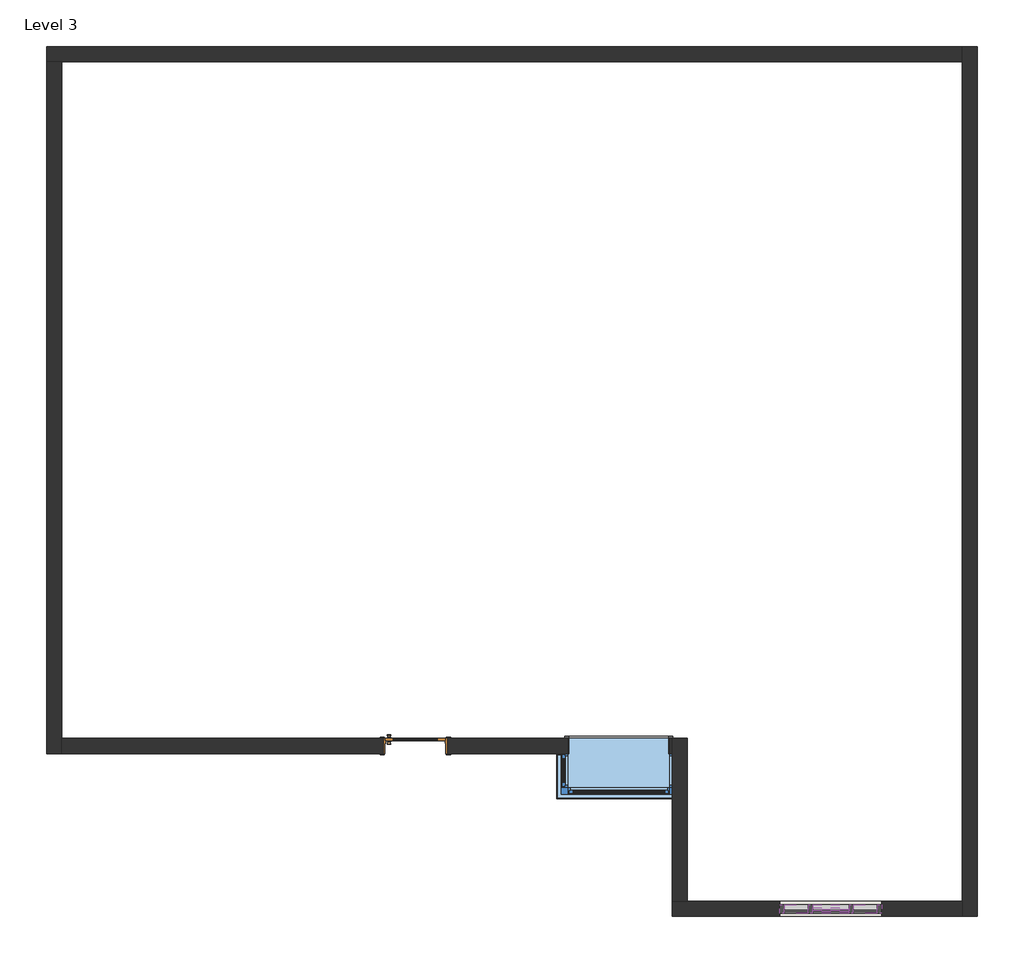
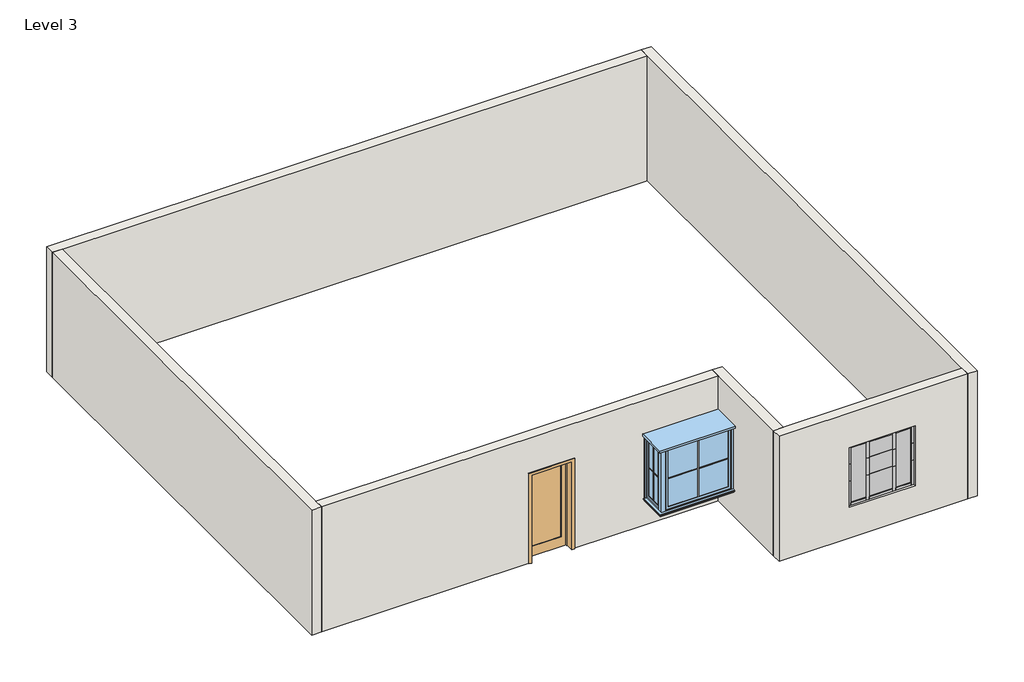
# One storey: 20 members, 6 walls, 5 plates, 4 proxies, 1 door, 1 window.
"""IFC4 building model written with IfcOpenShell, lengths in millimetres."""

from ifc_helpers import new_model, si_unit, origin, place, context, project, spatial, faceted_brep, transform, mapped, element, save
from components import muntin_pattern_2x2_muntin_pattern_2x2_eeef18e2, muntin_pattern_2x2_muntin_pattern_2x2_218eda85, trim_window_interior_flat_picture_frame_524b5c54, door_3b97b8e7, member_11e54509, member_471b44ca, member_576e3203, member_843225dc, member_a980948f, member_94122dd8, member_cc20b924, member_663db4d7, member_56ec01f9, system_panel_glazed_09ca6336, system_panel_glazed_ec18a58b, system_panel_glazed_fdb755d2, system_panel_glazed_b66c72d1, window_dda79932

model = new_model("IFC4")

# Units and contexts
model_context = context("Model", 3, world=origin())
ifc_project = project(units=[si_unit("LENGTHUNIT", "METRE", prefix="MILLI")], contexts=[model_context])

# Site, building, storey
site = spatial("IfcSite", under=ifc_project)
building = spatial("IfcBuilding", under=site)
storey = spatial("IfcBuildingStorey", under=building, Name="Level 3", Elevation=3810.0)

# Proxies
placement = place(None, origin())
muntin_pattern_2x2_muntin_pattern_2x2_shape = muntin_pattern_2x2_muntin_pattern_2x2_eeef18e2(model_context)
element("IfcBuildingElementProxy", 1, Name="Muntin Pattern_2x2 : Muntin Pattern_2x2", ObjectType="Muntin Pattern_2x2 : Muntin Pattern_2x2", at=placement, inside=storey, context=model_context, shape_type="MappedRepresentation", body=[
    mapped(muntin_pattern_2x2_muntin_pattern_2x2_shape, transform((2185.5135732, 136.9515264, 4540.25), x_axis=(-1.0, 0.0, 0.0), y_axis=(0.0, -1.0, 0.0), z_axis=(0.0, 0.0, 1.0))),
])
muntin_pattern_2x2_muntin_pattern_2x2_2_shape = muntin_pattern_2x2_muntin_pattern_2x2_218eda85(model_context)
element("IfcBuildingElementProxy", 2, Name="Muntin Pattern_2x2 : Muntin Pattern_2x2", ObjectType="Muntin Pattern_2x2 : Muntin Pattern_2x2", at=placement, inside=storey, context=model_context, shape_type="MappedRepresentation", body=[
    mapped(muntin_pattern_2x2_muntin_pattern_2x2_2_shape, transform((3007.8385732, 451.2765264, 4540.25), x_axis=(0.0, 1.0, 0.0), y_axis=(-1.0, 0.0, 0.0), z_axis=(0.0, 0.0, 1.0))),
])
element("IfcBuildingElementProxy", 3, Name="Muntin Pattern_2x2 : Muntin Pattern_2x2", ObjectType="Muntin Pattern_2x2 : Muntin Pattern_2x2", at=placement, inside=storey, context=model_context, shape_type="MappedRepresentation", body=[
    mapped(muntin_pattern_2x2_muntin_pattern_2x2_2_shape, transform((1363.1885732, 451.2765264, 4540.25), x_axis=(0.0, -1.0, 0.0), y_axis=(1.0, 0.0, 0.0), z_axis=(0.0, 0.0, 1.0))),
])
trim_window_interior_flat_picture_frame_shape = trim_window_interior_flat_picture_frame_524b5c54(model_context)
element("IfcBuildingElementProxy", 4, Name="Trim-Window-Interior-Flat : Picture Frame", ObjectType="Trim-Window-Interior-Flat : Picture Frame", at=placement, inside=storey, context=model_context, shape_type="MappedRepresentation", body=[
    mapped(trim_window_interior_flat_picture_frame_shape, transform((2185.5135732, 933.8765264, 5994.4), x_axis=(-1.0, 0.0, 0.0), y_axis=(0.0, 0.0, 1.0), z_axis=(0.0, 1.0, 0.0))),
])

# Door
door_shape = door_3b97b8e7(model_context)
element("IfcDoor", 5, ObjectType="Door-Interior-Single-1_Panel-Wood : 36\" x 84\"", at=placement, inside=storey, context=model_context, shape_type="MappedRepresentation", body=[
    mapped(door_shape, transform((-862.4864268, 822.7515264, 3810.0), x_axis=(1.0, 0.0, 0.0), y_axis=(0.0, 1.0, 0.0), z_axis=(0.0, 0.0, 1.0))),
])

# Members
member_shape = member_11e54509(model_context)
element("IfcMember", 6, ObjectType="Rectangular Mullion : 1\" Square", at=placement, inside=storey, context=model_context, shape_type="MappedRepresentation", body=[
    mapped(member_shape, transform((5087.4635732, -1618.8234736, 5573.6208294), x_axis=(0.0, 0.0, 1.0), y_axis=(0.0, 1.0, 0.0), z_axis=(-1.0, 0.0, 0.0))),
])
element("IfcMember", 7, ObjectType="Rectangular Mullion : 1\" Square", at=placement, inside=storey, context=model_context, shape_type="MappedRepresentation", body=[
    mapped(member_shape, transform((5087.4635732, -1618.8234736, 5158.7541627), x_axis=(0.0, 0.0, 1.0), y_axis=(0.0, 1.0, 0.0), z_axis=(-1.0, 0.0, 0.0))),
])
member_2_shape = member_471b44ca(model_context)
element("IfcMember", 8, ObjectType="Rectangular Mullion : 2.5\" x 5\" rectangular", at=placement, inside=storey, context=model_context, shape_type="MappedRepresentation", body=[
    mapped(member_2_shape, transform((5055.7135732, -1618.8234736, 5158.7541627), x_axis=(-1.0, 0.0, 0.0), y_axis=(0.0, 1.0, 0.0), z_axis=(0.0, 0.0, -1.0))),
])
element("IfcMember", 9, ObjectType="Rectangular Mullion : 2.5\" x 5\" rectangular", at=placement, inside=storey, context=model_context, shape_type="MappedRepresentation", body=[
    mapped(member_2_shape, transform((5665.3135732, -1618.8234736, 5158.7541627), x_axis=(-1.0, 0.0, 0.0), y_axis=(0.0, 1.0, 0.0), z_axis=(0.0, 0.0, -1.0))),
])
member_3_shape = member_576e3203(model_context)
element("IfcMember", 10, ObjectType="Rectangular Mullion : 2.5\" x 5\" rectangular", at=placement, inside=storey, context=model_context, shape_type="MappedRepresentation", body=[
    mapped(member_3_shape, transform((5055.7135732, -1618.8234736, 4557.6208294), x_axis=(-1.0, 0.0, 0.0), y_axis=(0.0, 1.0, 0.0), z_axis=(0.0, 0.0, -1.0))),
])
element("IfcMember", 11, ObjectType="Rectangular Mullion : 2.5\" x 5\" rectangular", at=placement, inside=storey, context=model_context, shape_type="MappedRepresentation", body=[
    mapped(member_3_shape, transform((5665.3135732, -1618.8234736, 4557.6208294), x_axis=(-1.0, 0.0, 0.0), y_axis=(0.0, 1.0, 0.0), z_axis=(0.0, 0.0, -1.0))),
])
member_4_shape = member_843225dc(model_context)
element("IfcMember", 12, ObjectType="Rectangular Mullion : 2.5\" x 5\" rectangular", at=placement, inside=storey, context=model_context, shape_type="MappedRepresentation", body=[
    mapped(member_4_shape, transform((4662.0135732, -1618.8234736, 6018.3521861), x_axis=(0.0, 0.0, 1.0), y_axis=(0.0, 1.0, 0.0), z_axis=(-1.0, 0.0, 0.0))),
])
element("IfcMember", 13, ObjectType="Rectangular Mullion : 2.5\" x 5\" rectangular", at=placement, inside=storey, context=model_context, shape_type="MappedRepresentation", body=[
    mapped(member_4_shape, transform((5697.0635732, -1618.8234736, 6018.3521861), x_axis=(0.0, 0.0, 1.0), y_axis=(0.0, 1.0, 0.0), z_axis=(-1.0, 0.0, 0.0))),
])
element("IfcMember", 14, ObjectType="Rectangular Mullion : 2.5\" x 5\" rectangular", at=placement, inside=storey, context=model_context, shape_type="MappedRepresentation", body=[
    mapped(member_4_shape, transform((6059.0135732, -1618.8234736, 4557.6208294), x_axis=(0.0, 0.0, -1.0), y_axis=(0.0, 1.0, 0.0), z_axis=(1.0, 0.0, 0.0))),
])
element("IfcMember", 15, ObjectType="Rectangular Mullion : 2.5\" x 5\" rectangular", at=placement, inside=storey, context=model_context, shape_type="MappedRepresentation", body=[
    mapped(member_4_shape, transform((5023.9635732, -1618.8234736, 4557.6208294), x_axis=(0.0, 0.0, -1.0), y_axis=(0.0, 1.0, 0.0), z_axis=(1.0, 0.0, 0.0))),
])
member_5_shape = member_a980948f(model_context)
element("IfcMember", 16, ObjectType="Rectangular Mullion : 2.5\" x 5\" rectangular", at=placement, inside=storey, context=model_context, shape_type="MappedRepresentation", body=[
    mapped(member_5_shape, transform((5633.5635732, -1618.8234736, 4557.6208294), x_axis=(0.0, 0.0, -1.0), y_axis=(0.0, 1.0, 0.0), z_axis=(1.0, 0.0, 0.0))),
])
element("IfcMember", 17, ObjectType="Rectangular Mullion : 2.5\" x 5\" rectangular", at=placement, inside=storey, context=model_context, shape_type="MappedRepresentation", body=[
    mapped(member_5_shape, transform((5087.4635732, -1618.8234736, 6018.3521861), x_axis=(0.0, 0.0, 1.0), y_axis=(0.0, 1.0, 0.0), z_axis=(-1.0, 0.0, 0.0))),
])
member_6_shape = member_94122dd8(model_context)
element("IfcMember", 18, ObjectType="Rectangular Mullion : 2.5\" x 5\" rectangular", at=placement, inside=storey, context=model_context, shape_type="MappedRepresentation", body=[
    mapped(member_6_shape, transform((4598.5135732, -1618.8234736, 4557.6208294), x_axis=(-1.0, 0.0, 0.0), y_axis=(0.0, 1.0, 0.0), z_axis=(0.0, 0.0, -1.0))),
])
member_7_shape = member_cc20b924(model_context)
element("IfcMember", 19, ObjectType="Rectangular Mullion : 2.5\" x 5\" rectangular", at=placement, inside=storey, context=model_context, shape_type="MappedRepresentation", body=[
    mapped(member_7_shape, transform((4598.5135732, -1618.8234736, 5158.7541627), x_axis=(-1.0, 0.0, 0.0), y_axis=(0.0, 1.0, 0.0), z_axis=(0.0, 0.0, -1.0))),
])
element("IfcMember", 20, ObjectType="Rectangular Mullion : 2.5\" x 5\" rectangular", at=placement, inside=storey, context=model_context, shape_type="MappedRepresentation", body=[
    mapped(member_7_shape, transform((6122.5135732, -1618.8234736, 5573.6208294), x_axis=(1.0, 0.0, 0.0), y_axis=(0.0, 1.0, 0.0), z_axis=(0.0, 0.0, 1.0))),
])
element("IfcMember", 21, ObjectType="Rectangular Mullion : 2.5\" x 5\" rectangular", at=placement, inside=storey, context=model_context, shape_type="MappedRepresentation", body=[
    mapped(member_6_shape, transform((6122.5135732, -1618.8234736, 5158.7541627), x_axis=(1.0, 0.0, 0.0), y_axis=(0.0, 1.0, 0.0), z_axis=(0.0, 0.0, 1.0))),
])
member_8_shape = member_663db4d7(model_context)
element("IfcMember", 22, ObjectType="Rectangular Mullion : 2.5\" x 5\" rectangular", at=placement, inside=storey, context=model_context, shape_type="MappedRepresentation", body=[
    mapped(member_8_shape, transform((5055.7135732, -1618.8234736, 5573.6208294), x_axis=(-1.0, 0.0, 0.0), y_axis=(0.0, 1.0, 0.0), z_axis=(0.0, 0.0, -1.0))),
])
element("IfcMember", 23, ObjectType="Rectangular Mullion : 2.5\" x 5\" rectangular", at=placement, inside=storey, context=model_context, shape_type="MappedRepresentation", body=[
    mapped(member_8_shape, transform((5665.3135732, -1618.8234736, 5573.6208294), x_axis=(-1.0, 0.0, 0.0), y_axis=(0.0, 1.0, 0.0), z_axis=(0.0, 0.0, -1.0))),
])
member_9_shape = member_56ec01f9(model_context)
element("IfcMember", 24, ObjectType="Rectangular Mullion : 2.5\" x 5\" rectangular", at=placement, inside=storey, context=model_context, shape_type="MappedRepresentation", body=[
    mapped(member_9_shape, transform((6122.5135732, -1618.8234736, 6018.3521861), x_axis=(1.0, 0.0, 0.0), y_axis=(0.0, 1.0, 0.0), z_axis=(0.0, 0.0, 1.0))),
])
element("IfcMember", 25, ObjectType="Rectangular Mullion : 2.5\" x 5\" rectangular", at=placement, inside=storey, context=model_context, shape_type="MappedRepresentation", body=[
    mapped(member_9_shape, transform((4598.5135732, -1618.8234736, 5573.6208294), x_axis=(-1.0, 0.0, 0.0), y_axis=(0.0, 1.0, 0.0), z_axis=(0.0, 0.0, -1.0))),
])

# Plates
system_panel_glazed_shape = system_panel_glazed_09ca6336(model_context)
element("IfcPlate", 26, ObjectType="System Panel : Glazed", at=placement, inside=storey, context=model_context, shape_type="MappedRepresentation", body=[
    mapped(system_panel_glazed_shape, transform((5360.5135732, -1618.8234736, 5158.7541627), x_axis=(-1.0, 0.0, 0.0), y_axis=(0.0, -1.0, 0.0), z_axis=(0.0, 0.0, 1.0))),
])
system_panel_glazed_2_shape = system_panel_glazed_ec18a58b(model_context)
element("IfcPlate", 27, ObjectType="System Panel : Glazed", at=placement, inside=storey, context=model_context, shape_type="MappedRepresentation", body=[
    mapped(system_panel_glazed_2_shape, transform((5360.5135732, -1618.8234736, 4621.1208294), x_axis=(-1.0, 0.0, 0.0), y_axis=(0.0, -1.0, 0.0), z_axis=(0.0, 0.0, 1.0))),
])
system_panel_glazed_3_shape = system_panel_glazed_fdb755d2(model_context)
element("IfcPlate", 28, ObjectType="System Panel : Glazed", at=placement, inside=storey, context=model_context, shape_type="MappedRepresentation", body=[
    mapped(system_panel_glazed_3_shape, transform((5878.0385732, -1618.8234736, 4621.1208294), x_axis=(-1.0, 0.0, 0.0), y_axis=(0.0, -1.0, 0.0), z_axis=(0.0, 0.0, 1.0))),
])
element("IfcPlate", 29, ObjectType="System Panel : Glazed", at=placement, inside=storey, context=model_context, shape_type="MappedRepresentation", body=[
    mapped(system_panel_glazed_3_shape, transform((4842.9885732, -1618.8234736, 4621.1208294), x_axis=(-1.0, 0.0, 0.0), y_axis=(0.0, -1.0, 0.0), z_axis=(0.0, 0.0, 1.0))),
])
system_panel_glazed_4_shape = system_panel_glazed_b66c72d1(model_context)
element("IfcPlate", 30, ObjectType="System Panel : Glazed", at=placement, inside=storey, context=model_context, shape_type="MappedRepresentation", body=[
    mapped(system_panel_glazed_4_shape, transform((5360.5135732, -1618.8234736, 5573.6208294), x_axis=(-1.0, 0.0, 0.0), y_axis=(0.0, -1.0, 0.0), z_axis=(0.0, 0.0, 1.0))),
])

# Walls
element("IfcWall", 31, ObjectType="9\" wall", at=placement, inside=storey, context=model_context, shape_type="Brep", body=[
    faceted_brep([(-6386.9864268, 11068.4765264, 3810.0), (-6158.3864268, 11068.4765264, 3810.0), (7329.0135732, 11068.4765264, 3810.0), (7329.0135732, 11068.4765264, 6858.0), (-6158.3864268, 11068.4765264, 6858.0), (-6386.9864268, 11068.4765264, 6858.0), (-6386.9864268, 11297.0765264, 3810.0), (-6386.9864268, 11297.0765264, 6858.0), (7329.0135732, 11297.0765264, 6858.0), (7329.0135732, 11297.0765264, 3810.0)], [[[0, 1, 2, 3, 4, 5]], [[6, 7, 8, 9]], [[2, 1, 0, 6, 9]], [[0, 5, 7, 6]], [[3, 2, 9, 8]], [[5, 4, 3, 8, 7]]]),
])
element("IfcWall", 32, ObjectType="9\" wall", at=placement, inside=storey, context=model_context, shape_type="Brep", body=[
    faceted_brep([(-6158.3864268, 705.2765264, 3810.0), (-6158.3864268, 933.8765264, 3810.0), (-6158.3864268, 11068.4765264, 3810.0), (-6158.3864268, 11068.4765264, 6858.0), (-6158.3864268, 933.8765264, 6858.0), (-6158.3864268, 705.2765264, 6858.0), (-6386.9864268, 705.2765264, 3810.0), (-6386.9864268, 705.2765264, 6858.0), (-6386.9864268, 11068.4765264, 6858.0), (-6386.9864268, 11068.4765264, 3810.0)], [[[0, 1, 2, 3, 4, 5]], [[6, 7, 8, 9]], [[2, 1, 0, 6, 9]], [[0, 5, 7, 6]], [[3, 2, 9, 8]], [[5, 4, 3, 8, 7]]]),
])
element("IfcWall", 33, ObjectType="9\" wall", at=placement, inside=storey, context=model_context, shape_type="Brep", body=[
    faceted_brep([(7329.0135732, 11297.0765264, 3810.0), (7329.0135732, 11068.4765264, 3810.0), (7329.0135732, -1504.5234736, 3810.0), (7329.0135732, -1733.1234736, 3810.0), (7329.0135732, -1733.1234736, 6858.0), (7329.0135732, -1504.5234736, 6858.0), (7329.0135732, 11068.4765264, 6858.0), (7329.0135732, 11297.0765264, 6858.0), (7557.6135732, 11297.0765264, 3810.0), (7557.6135732, 11297.0765264, 6858.0), (7557.6135732, -1733.1234736, 6858.0), (7557.6135732, -1733.1234736, 3810.0)], [[[0, 1, 2, 3, 4, 5, 6, 7]], [[8, 9, 10, 11]], [[3, 2, 1, 0, 8, 11]], [[0, 7, 9, 8]], [[4, 3, 11, 10]], [[7, 6, 5, 4, 10, 9]]]),
])
element("IfcWall", 34, ObjectType="9\" wall", at=placement, inside=storey, context=model_context, shape_type="Brep", body=[
    faceted_brep([(7329.0135732, -1504.5234736, 3810.0), (3214.2135732, -1504.5234736, 3810.0), (2985.6135732, -1504.5234736, 3810.0), (2985.6135732, -1504.5234736, 6858.0), (3214.2135732, -1504.5234736, 6858.0), (7329.0135732, -1504.5234736, 6858.0), (6122.5135732, -1504.5234736, 4557.6208294), (6122.5135732, -1504.5234736, 6018.3521861), (4598.5135732, -1504.5234736, 6018.3521861), (4598.5135732, -1504.5234736, 4557.6208294), (2985.6135732, -1733.1234736, 3810.0), (7329.0135732, -1733.1234736, 3810.0), (7329.0135732, -1733.1234736, 6858.0), (2985.6135732, -1733.1234736, 6858.0), (6122.5135732, -1733.1234736, 6018.3521861), (6122.5135732, -1733.1234736, 4557.6208294), (4598.5135732, -1733.1234736, 4557.6208294), (4598.5135732, -1733.1234736, 6018.3521861)], [[[0, 1, 2, 3, 4, 5], [6, 7, 8, 9]], [[10, 11, 12, 13], [14, 15, 16, 17]], [[2, 1, 0, 11, 10]], [[0, 5, 12, 11]], [[3, 2, 10, 13]], [[6, 15, 14, 7]], [[7, 14, 17, 8]], [[8, 17, 16, 9]], [[15, 6, 9, 16]], [[5, 4, 3, 13, 12]]]),
])
element("IfcWall", 35, ObjectType="9\" wall", at=placement, inside=storey, context=model_context, shape_type="Brep", body=[
    faceted_brep([(3214.2135732, -1504.5234736, 3810.0), (3214.2135732, 933.8765264, 3810.0), (3214.2135732, 933.8765264, 6858.0), (3214.2135732, -1504.5234736, 6858.0), (2985.6135732, -1504.5234736, 3810.0), (2985.6135732, -1504.5234736, 6858.0), (2985.6135732, 705.2765264, 6858.0), (2985.6135732, 933.8765264, 6858.0), (2985.6135732, 933.8765264, 3810.0), (2985.6135732, 705.2765264, 3810.0)], [[[0, 1, 2, 3]], [[4, 5, 6, 7, 8, 9]], [[1, 0, 4, 9, 8]], [[0, 3, 5, 4]], [[2, 1, 8, 7]], [[3, 2, 7, 6, 5]]]),
])
element("IfcWall", 36, ObjectType="9\" wall", at=placement, inside=storey, context=model_context, shape_type="Brep", body=[
    faceted_brep([(-6158.3864268, 933.8765264, 3810.0), (-6158.3864268, 933.8765264, 6858.0), (2985.6135732, 933.8765264, 6858.0), (2985.6135732, 933.8765264, 3810.0), (-379.8864268, 933.8765264, 3810.0), (-379.8864268, 933.8765264, 5969.0), (-1345.0864268, 933.8765264, 5969.0), (-1345.0864268, 933.8765264, 3810.0), (1423.5135732, 933.8765264, 5994.4), (1423.5135732, 933.8765264, 4419.6), (2947.5135732, 933.8765264, 4419.6), (2947.5135732, 933.8765264, 5994.4), (-6158.3864268, 705.2765264, 6858.0), (-6158.3864268, 705.2765264, 3810.0), (-1345.0864268, 705.2765264, 3810.0), (-1345.0864268, 705.2765264, 5969.0), (-379.8864268, 705.2765264, 5969.0), (-379.8864268, 705.2765264, 3810.0), (2985.6135732, 705.2765264, 3810.0), (2985.6135732, 705.2765264, 6858.0), (365.6851234, 705.2765264, 6858.0), (1423.5135732, 705.2765264, 4419.6), (1423.5135732, 705.2765264, 5994.4), (2947.5135732, 705.2765264, 5994.4), (2947.5135732, 705.2765264, 4419.6)], [[[0, 1, 2, 3, 4, 5, 6, 7], [8, 9, 10, 11]], [[12, 13, 14, 15, 16, 17, 18, 19, 20], [21, 22, 23, 24]], [[13, 0, 7, 14]], [[3, 18, 17, 4]], [[1, 0, 13, 12]], [[3, 2, 19, 18]], [[9, 8, 22, 21]], [[10, 9, 21, 24]], [[11, 10, 24, 23]], [[8, 11, 23, 22]], [[19, 2, 1, 12, 20]], [[16, 5, 4, 17]], [[5, 16, 15, 6]], [[6, 15, 14, 7]]]),
])

# Window
window_shape = window_dda79932(model_context)
element("IfcWindow", 37, ObjectType="Window-Bay-Casement-Box-90_Degree_Angle-Center_Fixed : 60\" x 60\" x 24\"", at=placement, inside=storey, context=model_context, shape_type="MappedRepresentation", body=[
    mapped(window_shape, transform((2185.5135732, 819.5765264, 3810.0), x_axis=(-1.0, 0.0, 0.0), y_axis=(0.0, -1.0, 0.0), z_axis=(0.0, 0.0, 1.0))),
])

save(model, "model.ifc")

# Revit data of these elements
# Type "Muntin Pattern_2x2 : Muntin Pattern_2x2"
#   Width [instance default] = 4' - 0"
#   Thickness = 0' - 0 1/2"
#   Height [instance default] = 4' - 0"
#   Distance = 0' - 0 3/4"
#   Interior Material [instance default] = none
#   Exterior Material [instance default] = none
#   Default Elevation = 0
# Type "Trim-Window-Interior-Flat : Picture Frame"
#   Trim Thickness_Picture Frame = 0' - 1 1/4"
#   Trim Width = 0' - 2 1/4"
#   Trim Thickness_with Sill = 0' - 0 3/4"
#   Sill Thickness = 0' - 1 1/4"
#   Opening Width [instance default] = 2' - 0"
#   Opening Height [instance default] = 3' - 0"
#   Default Elevation = 4' - 0"
#   Sill = no
#   Picture Frame = yes
#   Trim Material [instance default] = none
# Type "Door-Interior-Single-1_Panel-Wood : 36\" x 84\""
#   Type Mark = "8"
#   Assembly Code = "C1020300"
#   Analytic Construction = "Wooden"
#   Top Rail = 0' - 4 11/16"
#   Thickness = 0' - 1 3/8"
#   Thermal Resistance (R) = 2.5876 (h·ft²·°F)/BTU
#   Swing Angle [instance default] = 90.00°
#   Stiles = 0' - 4 3/4"
#   Rough Width = 3' - 2"
#   Rough Height = 7' - 1"
#   Height = 7' - 0"
#   Width = 3' - 0"
#   Heat Transfer Coefficient (U) = 0.3865 BTU/(h·ft²·°F)
#   Bottom Rail = 0' - 9 1/8"
#   Trim Material = Cherry
#   Panel Material = Cherry
#   Frame Material = Cherry
#   Door Handle Material = Aluminum
#   Visual Light Transmittance = 0
#   Solar Heat Gain Coefficient = 0
#   Wall Closure = (empty or 0)
#   Function = (empty or 0)
# Type "Rectangular Mullion : 1\" Square"
#   built-in parameter 1007350 = 0.0416667 (stored number, unit not read)
# Type "Rectangular Mullion : 2.5\" x 5\" rectangular"
#   built-in parameter 1007304 = 0.416667 (stored number, unit not read)
#   built-in parameter 1007301 = 0.104167 (stored number, unit not read)
#   built-in parameter 1007300 = 0.104167 (stored number, unit not read)
# Type "System Panel : Glazed"
#   Construction Type Id = "GSP4R"
#   Analytic Construction = "1/8 in Pilkington single glazing"
#   Visual Light Transmittance = 0.9
#   Solar Heat Gain Coefficient = 0.86
#   Heat Transfer Coefficient (U) = 1.18115 BTU/(h·ft²·°F)
#   Define Thermal Properties by = 1
# Type "9\" wall"
#   Assembly Code = "B2010"
#   Layers, outside or top first: 0' - 9" "wall" (function 1)
# Type "Window-Bay-Casement-Box-90_Degree_Angle-Center_Fixed : 60\" x 60\" x 24\""
#   Type Mark = "18"
#   Fire Rating = "0.5h"
#   Assembly Code = "B2020100"
#   Analytic Construction = "1/8 in Pilkington single glazing"
#   Width = 5' - 0"
#   Wall Thickness [instance default] = 0' - 6"
#   Visual Light Transmittance = 0.9
#   Trim Width = 5' - 8"
#   Trim Height = 5' - 0"
#   Thermal Resistance (R) = 1.5394 (h·ft²·°F)/BTU
#   Solar Heat Gain Coefficient = 0.86
#   Rough Width = 5' - 0 1/2"
#   Rough Height = 5' - 0 1/2"
#   Height 1 = 5' - 2"
#   Height = 5' - 0"
#   Heat Transfer Coefficient (U) = 0.6496 BTU/(h·ft²·°F)
#   Depth = 2' - 0"
#   Default Sill Height = 2' - 0"
#   Side Muntin Visibility = yes
#   Center Muntin Visibility = yes
#   Interior Trim Visibility [instance default] = yes
#   Exterior Trim Visibility [instance default] = yes
#   Side Muntin Pattern = Muntin Pattern_2x2 : Muntin Pattern_2x2
#   Center Muntin Pattern = Muntin Pattern_2x2 : Muntin Pattern_2x2
#   Interior Trim Material = Wood - Stained
#   Exterior Trim Material = Clad - White
#   Exterior Trim = element 385931
#   Interior Trim = Trim-Window-Interior-Flat : Picture Frame
#   Interior Frame Material = Wood - Stained
#   Glass Panel Material = Glass
#   Exterior Frame Material = Clad - White
#   Wall Closure = (empty or 0)
# Element 1 (IfcBuildingElementProxy, "Muntin Pattern_2x2 : Muntin Pattern_2x2")
#   Width = 4' - 6 1/2"
#   Height = 4' - 6 1/2"
#   Interior Material = Wood - Stained
#   Exterior Material = Clad - White
#   Phase Created = New Construction
#   Materials on its faces: "Clad - White", "Wood - Stained"
# Elements 2, 3 (IfcBuildingElementProxy, "Muntin Pattern_2x2 : Muntin Pattern_2x2")
#   Width = 1' - 2 1/2"
#   Height = 4' - 6 1/2"
#   Interior Material = Wood - Stained
#   Exterior Material = Clad - White
#   Phase Created = New Construction
#   Materials on its faces: "Clad - White", "Wood - Stained"
# Element 4 (IfcBuildingElementProxy, "Trim-Window-Interior-Flat : Picture Frame")
#   Opening Width = 5' - 0"
#   Opening Height = 5' - 2"
#   Trim Material = Wood - Stained
#   Phase Created = New Construction
#   Materials on its faces: "Wood - Stained"
# Element 5 (IfcDoor, "Door-Interior-Single-1_Panel-Wood : 36\" x 84\"")
#   Swing Angle = 90.00°
#   Phase Created = New Construction
#   Materials on its faces: "Cherry", "Aluminum"
# Elements 6, 7 (IfcMember, "Rectangular Mullion : 1\" Square")
#   Phase Created = New Construction
#   Materials on its faces: "Aluminum"
# Elements 8, 9, 10, 11, 12, 13, 14, 15, 16, 17, 18, 19, 20, 21, 22, 23, 24, 25 (IfcMember, "Rectangular Mullion : 2.5\" x 5\" rectangular")
#   Phase Created = New Construction
#   Materials on its faces: "Aluminum"
# Elements 26, 27, 28, 29, 30 (IfcPlate, "System Panel : Glazed")
#   Phase Created = New Construction
#   Materials on its faces: "Glass"
# Elements 31, 32, 33, 34, 35, 36 (IfcWall, "9\" wall")
#   Top Offset = 0' - 0"
#   Base Offset = 0' - 0"
#   wall height = 10' - 0"
#   Phase Created = New Construction
#   Base Constraint = Level 3
#   Top Constraint = Level 4
#   Materials on its faces: "wall"
# Element 37 (IfcWindow, "Window-Bay-Casement-Box-90_Degree_Angle-Center_Fixed : 60\" x 60\" x 24\"")
#   Mark = "1"
#   Interior Trim Visibility = yes
#   Exterior Trim Visibility = yes
#   Phase Created = New Construction
#   Materials on its faces: "Clad - White", "Wood - Stained", "Glass"
# Materials
#   "Cherry": class "Wood", colour RGB 226 177 128, transparency 0, Description = "Prunus Serotina", Cost = 0
#   "Aluminum": class "Metal", colour RGB 247 247 247, transparency 0, Description = "Aluminum 6061", Cost = 0
#   "wall": class "Generic", colour RGB 120 120 120, transparency 0, Cost = 0
#   "Wood - Stained": class "Wood", colour RGB 224 178 126, transparency 0, Cost = 0
#   "Clad - White": class "Wood", colour RGB 242 242 238, transparency 0, Cost = 0
#   "Glass": class "Glass", colour RGB 0 128 192, transparency 0.75, Description = "Soda Lime Glass", Cost = 0
